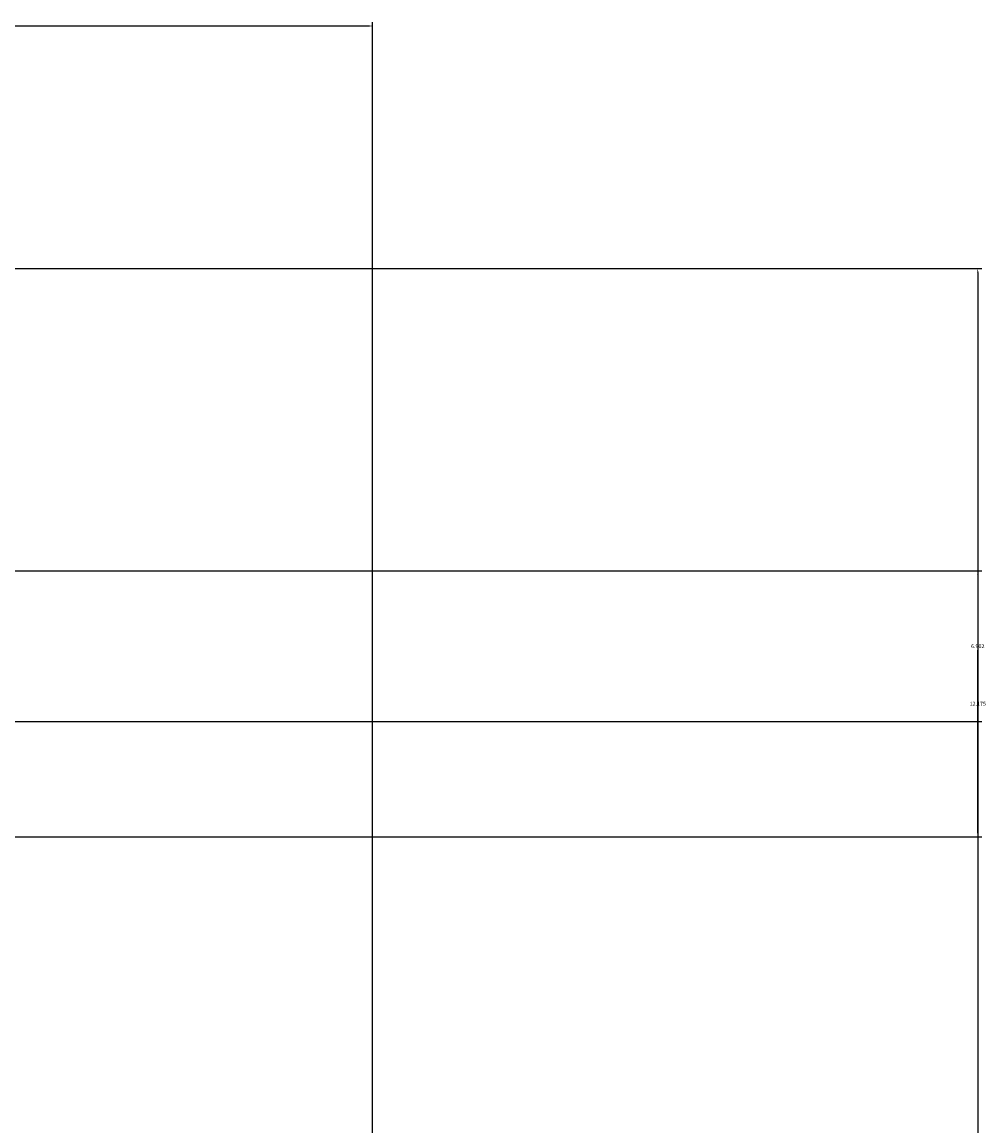
# Model space of a CAD drawing. Units: inches. Extents: x 412 to 584, y 208 to 437.
# Tile 28 of 28: x 540 to 584, y 387 to 437. Entities that reach past the tile are written whole.
import ezdxf

# ---------------------------------------------------------------- set-up
doc = ezdxf.new("R2010")
doc.units = ezdxf.units.IN
doc.header["$MEASUREMENT"] = 0
doc.layers.add('A-ANNO-DIMS', color=2, linetype='Continuous', lineweight=18)
doc.styles.get("Standard").update_dxf_attribs({"font": 'arial.ttf'})
doc.dimstyles.get("Standard").update_dxf_attribs({"dimtxt": 0.18, "dimasz": 0.18, "dimexe": 0.18, "dimexo": 0.0625, "dimgap": 0.09, "dimtad": 0, "dimtih": 1, "dimtoh": 1, "dimdec": 4, "dimzin": 0, "dimdsep": 46, "dimtxsty": 'Standard', "dimcen": 0.09, "dimadec": 0, "dimazin": 0, "dimtfac": 1, "dimtdec": 4, "dimtofl": 0, "dimtmove": 0, "dimatfit": 3, "dimfxl": 1, "dimtolj": 1, "dimtzin": 0, "dimarcsym": 0})

# ---------------------------------------------------------------- blocks, each defined once
blk = doc.blocks.new('*D17')
at = {"layer": 'A-ANNO-DIMS', "color": 0, "lineweight": -2, "transparency": 16777216}
for p, q in [((497.715, 426.185), (583.674, 426.185)), ((583.494, 426.005), (583.494, 323.031)), ((583.494, 219.693), (583.494, 322.667)), ((550.198, 219.513), (583.674, 219.513))]:
    blk.add_line(p, q, dxfattribs=at)
at = {"layer": 'A-ANNO-DIMS', "color": 0, "transparency": 16777216}
for points in [[(583.464, 426.005), (583.524, 426.005), (583.494, 426.185)], [(583.464, 219.693), (583.524, 219.693), (583.494, 219.513)]]:
    blk.add_solid(points, dxfattribs=at)
at = {"layer": 'Defpoints', "color": 0, "transparency": 16777216}
for p in [(497.652, 426.185), (550.135, 219.513), (583.494, 219.513)]:
    blk.add_point(p, dxfattribs=at)
at = {"layer": 'A-ANNO-DIMS', "color": 0, "transparency": 16777216, "insert": (583.494, 322.849), "char_height": 0.18, "attachment_point": 5}
blk.add_mtext('\\A1;206.67', dxfattribs=at)
blk = doc.blocks.new('*D20')
at = {"layer": 'A-ANNO-DIMS', "color": 0, "lineweight": -2, "transparency": 16777216}
for p, q in [((507.316, 412.35), (583.674, 412.35)), ((583.494, 412.17), (583.494, 406.444)), ((583.494, 400.355), (583.494, 406.08)), ((538.681, 400.175), (583.674, 400.175))]:
    blk.add_line(p, q, dxfattribs=at)
at = {"layer": 'A-ANNO-DIMS', "color": 0, "transparency": 16777216}
for points in [[(583.464, 412.17), (583.524, 412.17), (583.494, 412.35)], [(583.464, 400.355), (583.524, 400.355), (583.494, 400.175)]]:
    blk.add_solid(points, dxfattribs=at)
at = {"layer": 'Defpoints', "color": 0, "transparency": 16777216}
for p in [(507.254, 412.35), (538.619, 400.175), (583.494, 400.175)]:
    blk.add_point(p, dxfattribs=at)
at = {"layer": 'A-ANNO-DIMS', "color": 0, "transparency": 16777216, "insert": (583.494, 406.262), "char_height": 0.18, "attachment_point": 5}
blk.add_mtext('\\A1;12.175', dxfattribs=at)
blk = doc.blocks.new('*D28')
at = {"layer": 'A-ANNO-DIMS', "color": 0, "lineweight": -2, "transparency": 16777216}
for p, q in [((450.562, 256.635), (450.562, 437.465)), ((450.742, 437.285), (502.724, 437.285)), ((555.616, 437.285), (503.634, 437.285)), ((555.796, 256.635), (555.796, 437.465))]:
    blk.add_line(p, q, dxfattribs=at)
at = {"layer": 'A-ANNO-DIMS', "color": 0, "transparency": 16777216}
for points in [[(450.742, 437.315), (450.742, 437.255), (450.562, 437.285)], [(555.616, 437.315), (555.616, 437.255), (555.796, 437.285)]]:
    blk.add_solid(points, dxfattribs=at)
at = {"layer": 'Defpoints', "color": 0, "transparency": 16777216}
for p in [(555.796, 437.285), (450.562, 256.573), (555.796, 256.573)]:
    blk.add_point(p, dxfattribs=at)
at = {"layer": 'A-ANNO-DIMS', "color": 0, "transparency": 16777216, "insert": (503.179, 437.285), "char_height": 0.18, "attachment_point": 5}
blk.add_mtext('\\A1;105.23', dxfattribs=at)
blk = doc.blocks.new('*D32')
at = {"layer": 'A-ANNO-DIMS', "color": 0, "lineweight": -2, "transparency": 16777216}
for p, q in [((507.316, 412.35), (583.674, 412.35)), ((583.494, 412.17), (583.494, 409.081)), ((583.494, 405.628), (583.494, 408.717)), ((507.316, 405.448), (583.674, 405.448))]:
    blk.add_line(p, q, dxfattribs=at)
at = {"layer": 'A-ANNO-DIMS', "color": 0, "transparency": 16777216}
for points in [[(583.464, 412.17), (583.524, 412.17), (583.494, 412.35)], [(583.464, 405.628), (583.524, 405.628), (583.494, 405.448)]]:
    blk.add_solid(points, dxfattribs=at)
at = {"layer": 'Defpoints', "color": 0, "transparency": 16777216}
for p in [(507.254, 412.35), (507.254, 405.448), (583.494, 405.448)]:
    blk.add_point(p, dxfattribs=at)
at = {"layer": 'A-ANNO-DIMS', "color": 0, "transparency": 16777216, "insert": (583.494, 408.899), "char_height": 0.18, "attachment_point": 5}
blk.add_mtext('\\A1;6.902', dxfattribs=at)

msp = doc.modelspace()

# ---------------------------------------------------------------- dimensions: what is measured, and where the dimension line sits
at = {"layer": 'A-ANNO-DIMS'}
dim = msp.add_linear_dim(base=(555.7959, 437.2847), p1=(450.562, 256.5729), p2=(555.7959, 256.5729), dimstyle='Standard', override={"dimdec": 2, "dimlfac": 1, "dimrnd": 0, "dimzin": 0, "dimdsep": 46, "dimlunit": 2}, dxfattribs=at)
dim.commit()
dim.dimension.update_dxf_attribs({"geometry": '*D28', "text_midpoint": (503.1789, 437.2847)})
for base, p1, p2, override, picture, middle in [((583.4937, 219.5133), (497.6523, 426.1847), (550.1351, 219.5133), {"dimdec": 2, "dimlfac": 1, "dimrnd": 0, "dimzin": 0, "dimdsep": 46, "dimlunit": 2}, '*D17', (583.4937, 322.849)), ((583.4937, 400.175), (507.2538, 412.3496), (538.6186, 400.175), {"dimdec": 3, "dimlfac": 1, "dimrnd": 0, "dimzin": 0, "dimdsep": 46, "dimlunit": 2}, '*D20', (583.4937, 406.2623)), ((583.4937, 405.448), (507.2538, 412.3496), (507.2538, 405.448), {"dimdec": 3, "dimlfac": 1, "dimrnd": 0, "dimzin": 0, "dimdsep": 46, "dimlunit": 2}, '*D32', (583.4937, 408.8988))]:
    dim = msp.add_linear_dim(base=base, p1=p1, p2=p2, angle=90, dimstyle='Standard', override=override, dxfattribs=at)
    dim.commit()
    dim.dimension.update_dxf_attribs({"geometry": picture, "text_midpoint": middle})

doc.saveas('drawing.dxf')
